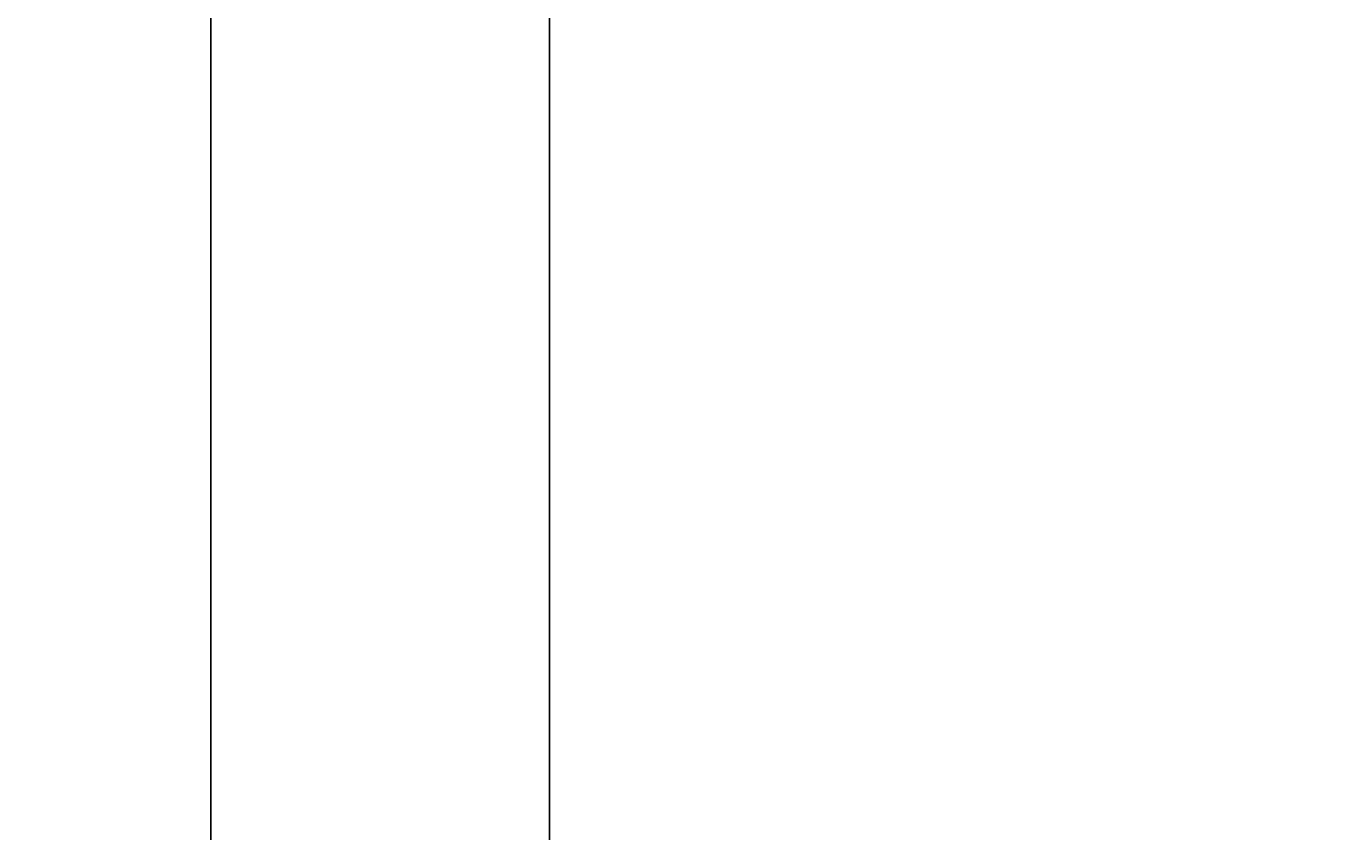
# Model space of a CAD drawing. Units: inches. Extents: x 35362 to 73946, y 43607 to 67532.
# Tile 72 of 134: x 47763 to 49302, y 49738 to 50677. Entities that reach past the tile are written whole.
import ezdxf

# ---------------------------------------------------------------- set-up
doc = ezdxf.new("R2010")
doc.units = ezdxf.units.IN
doc.header["$MEASUREMENT"] = 0
doc.layers.add('A-ANNO-DIMS', color=2, linetype='Continuous', lineweight=18)
doc.styles.get("Standard").update_dxf_attribs({"font": 'arial.ttf'})
doc.dimstyles.get("Standard").update_dxf_attribs({"dimtxt": 0.18, "dimasz": 0.18, "dimexe": 0.18, "dimexo": 0.0625, "dimgap": 0.09, "dimtad": 0, "dimtih": 1, "dimtoh": 1, "dimdec": 4, "dimzin": 0, "dimdsep": 46, "dimtxsty": 'Standard', "dimcen": 0.09, "dimadec": 0, "dimazin": 0, "dimtfac": 1, "dimtdec": 4, "dimtofl": 0, "dimtmove": 0, "dimatfit": 3, "dimfxl": 1, "dimtolj": 1, "dimtzin": 0, "dimarcsym": 0})

# ---------------------------------------------------------------- blocks, each defined once
blk = doc.blocks.new('*D11')
at = {"layer": 'A-ANNO-DIMS', "color": 0, "lineweight": -2, "transparency": 16777216}
for p, q in [((47978.7, 56028.8), (47978.7, 43606.7)), ((53109.8, 56028.8), (53109.8, 43606.7)), ((47978.8, 43606.9), (50543.9, 43606.9)), ((53109.6, 43606.9), (50544.6, 43606.9))]:
    blk.add_line(p, q, dxfattribs=at)
at = {"layer": 'A-ANNO-DIMS', "color": 0, "transparency": 16777216}
for points in [[(47978.8, 43606.9), (47978.8, 43606.8), (47978.7, 43606.9)], [(53109.6, 43606.9), (53109.6, 43606.8), (53109.8, 43606.9)]]:
    blk.add_solid(points, dxfattribs=at)
at = {"layer": 'Defpoints', "color": 0, "transparency": 16777216}
for p in [(47978.7, 56028.8), (53109.8, 56028.8), (53109.8, 43606.9)]:
    blk.add_point(p, dxfattribs=at)
at = {"layer": 'A-ANNO-DIMS', "color": 0, "transparency": 16777216, "insert": (50544.2, 43606.9), "char_height": 0.18, "attachment_point": 5}
blk.add_mtext('\\A1;5131', dxfattribs=at)
blk = doc.blocks.new('*D13')
at = {"layer": 'A-ANNO-DIMS', "color": 0, "lineweight": -2, "transparency": 16777216}
for p, q in [((48373.5, 51694), (48373.5, 43606.7)), ((51029, 51694), (51029, 43606.7)), ((48373.7, 43606.9), (49700.8, 43606.9)), ((51028.9, 43606.9), (49701.7, 43606.9))]:
    blk.add_line(p, q, dxfattribs=at)
at = {"layer": 'A-ANNO-DIMS', "color": 0, "transparency": 16777216}
for points in [[(48373.7, 43606.9), (48373.7, 43606.8), (48373.5, 43606.9)], [(51028.9, 43606.9), (51028.9, 43606.8), (51029, 43606.9)]]:
    blk.add_solid(points, dxfattribs=at)
at = {"layer": 'Defpoints', "color": 0, "transparency": 16777216}
for p in [(48373.5, 51694.1), (51029, 51694.1), (51029, 43606.9)]:
    blk.add_point(p, dxfattribs=at)
at = {"layer": 'A-ANNO-DIMS', "color": 0, "transparency": 16777216, "insert": (49701.3, 43606.9), "char_height": 0.18, "attachment_point": 5}
blk.add_mtext('\\A1;2655.6', dxfattribs=at)
blk = doc.blocks.new('*D27')
at = {"layer": 'A-ANNO-DIMS', "color": 0, "lineweight": -2, "transparency": 16777216}
for p, q in [((47978.7, 56028.8), (47978.7, 43606.7)), ((48373.5, 53429), (48373.5, 43606.7)), ((47978.8, 43606.9), (48175.7, 43606.9)), ((48373.3, 43606.9), (48176.5, 43606.9))]:
    blk.add_line(p, q, dxfattribs=at)
at = {"layer": 'A-ANNO-DIMS', "color": 0, "transparency": 16777216}
for points in [[(47978.8, 43606.9), (47978.8, 43606.8), (47978.7, 43606.9)], [(48373.3, 43606.9), (48373.3, 43606.8), (48373.5, 43606.9)]]:
    blk.add_solid(points, dxfattribs=at)
at = {"layer": 'Defpoints', "color": 0, "transparency": 16777216}
for p in [(47978.7, 56028.8), (48373.5, 53429), (48373.5, 43606.9)]:
    blk.add_point(p, dxfattribs=at)
at = {"layer": 'A-ANNO-DIMS', "color": 0, "transparency": 16777216, "insert": (48176.1, 43606.9), "char_height": 0.18, "attachment_point": 5}
blk.add_mtext('\\A1;394.8', dxfattribs=at)
blk = doc.blocks.new('*D40')
at = {"layer": 'A-ANNO-DIMS', "color": 0, "lineweight": -2, "transparency": 16777216}
for p, q in [((56873.5, 53351.5), (35361.8, 53351.5)), ((35361.9, 53351.3), (35361.9, 51333.3)), ((35361.9, 49314.8), (35361.9, 51332.9)), ((51806.5, 49314.7), (35361.8, 49314.7))]:
    blk.add_line(p, q, dxfattribs=at)
at = {"layer": 'A-ANNO-DIMS', "color": 0, "transparency": 16777216}
for points in [[(35361.9, 53351.3), (35362, 53351.3), (35361.9, 53351.5)], [(35361.9, 49314.8), (35362, 49314.8), (35361.9, 49314.7)]]:
    blk.add_solid(points, dxfattribs=at)
at = {"layer": 'Defpoints', "color": 0, "transparency": 16777216}
for p in [(35361.9, 53351.5), (56873.6, 53351.5), (51806.5, 49314.7)]:
    blk.add_point(p, dxfattribs=at)
at = {"layer": 'A-ANNO-DIMS', "color": 0, "transparency": 16777216, "insert": (35361.9, 51333.1), "char_height": 0.18, "attachment_point": 5}
blk.add_mtext('\\A1;4036.9', dxfattribs=at)
blk = doc.blocks.new('*D67')
at = {"layer": 'A-ANNO-DIMS', "color": 0, "lineweight": -2, "transparency": 16777216}
for p, q in [((56873.5, 53351.5), (35361.8, 53351.5)), ((35361.9, 53351.3), (35361.9, 49400.9)), ((35361.9, 45450.1), (35361.9, 49400.5)), ((53793.6, 45449.9), (35361.8, 45449.9))]:
    blk.add_line(p, q, dxfattribs=at)
at = {"layer": 'A-ANNO-DIMS', "color": 0, "transparency": 16777216}
for points in [[(35361.9, 53351.3), (35362, 53351.3), (35361.9, 53351.5)], [(35361.9, 45450.1), (35362, 45450.1), (35361.9, 45449.9)]]:
    blk.add_solid(points, dxfattribs=at)
at = {"layer": 'Defpoints', "color": 0, "transparency": 16777216}
for p in [(35361.9, 53351.5), (56873.6, 53351.5), (53793.6, 45449.9)]:
    blk.add_point(p, dxfattribs=at)
at = {"layer": 'A-ANNO-DIMS', "color": 0, "transparency": 16777216, "insert": (35361.9, 49400.7), "char_height": 0.18, "attachment_point": 5}
blk.add_mtext('\\A1;7901.6', dxfattribs=at)

msp = doc.modelspace()

# ---------------------------------------------------------------- dimensions: what is measured, and where the dimension line sits
at = {"layer": 'A-ANNO-DIMS'}
for base, p1, p2, override, picture, middle in [((53109.76, 43606.859), (47978.665, 56028.836), (53109.76, 56028.836), {"dimdec": 0, "dimlfac": 1, "dimrnd": 0, "dimzin": 0, "dimdsep": 46, "dimlunit": 2}, '*D11', (50544.212, 43606.859)), ((48373.492, 43606.859), (47978.665, 56028.836), (48373.492, 53429.019), {"dimdec": 1, "dimlfac": 1, "dimrnd": 0, "dimzin": 0, "dimdsep": 46, "dimlunit": 2}, '*D27', (48176.078, 43606.859)), ((51029.043, 43606.859), (48373.492, 51694.087), (51029.043, 51694.087), {"dimdec": 1, "dimlfac": 1, "dimrnd": 0, "dimzin": 0, "dimdsep": 46, "dimlunit": 2}, '*D13', (49701.267, 43606.859))]:
    dim = msp.add_linear_dim(base=base, p1=p1, p2=p2, dimstyle='Standard', override=override, dxfattribs=at)
    dim.commit()
    dim.dimension.update_dxf_attribs({"geometry": picture, "text_midpoint": middle})
for p1, picture, middle in [((51806.517, 49314.669), '*D40', (35361.949, 51333.099)), ((53793.638, 45449.894), '*D67', (35361.949, 49400.712))]:
    dim = msp.add_linear_dim(base=(35361.949, 53351.529), p1=p1, p2=(56873.602, 53351.529), angle=90, dimstyle='Standard', override={"dimdec": 1, "dimlfac": 1, "dimrnd": 0, "dimzin": 0, "dimdsep": 46, "dimlunit": 2}, dxfattribs=at)
    dim.commit()
    dim.dimension.update_dxf_attribs({"geometry": picture, "text_midpoint": middle})

doc.saveas('drawing.dxf')
